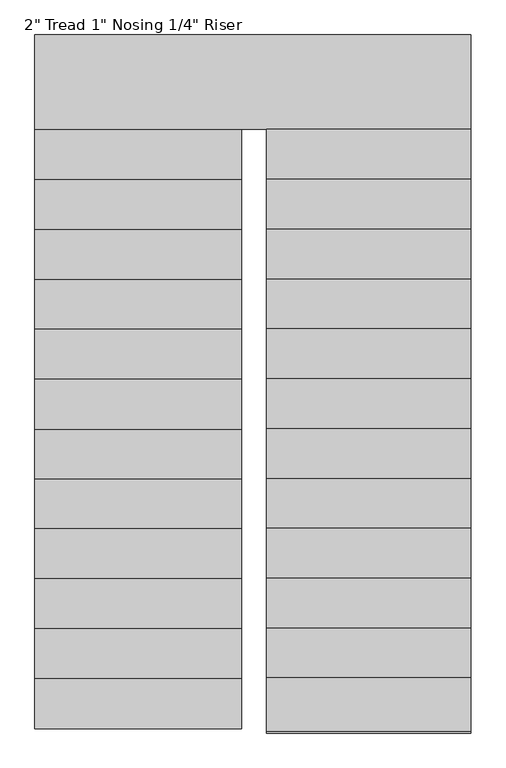
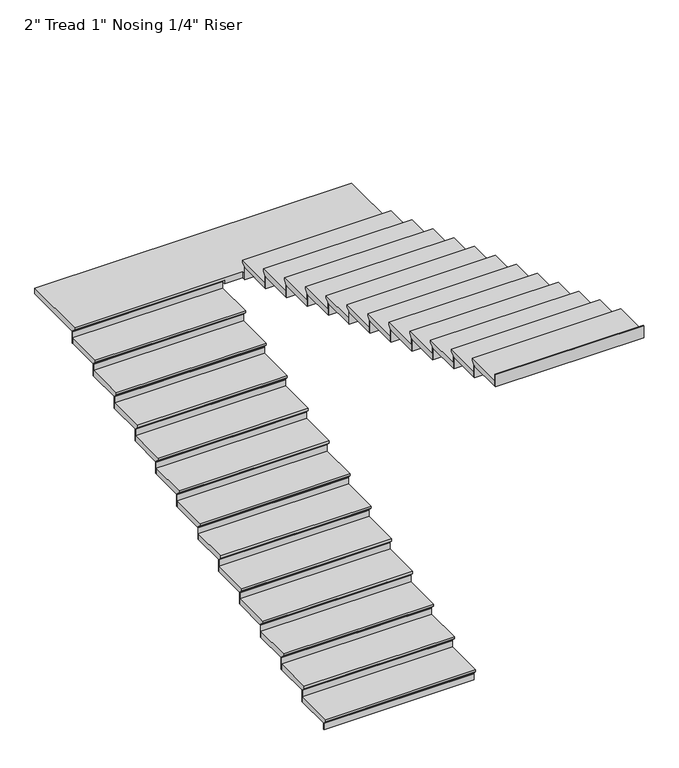
"""IFC4 building model written with IfcOpenShell, lengths in millimetres: stair flight geometry."""

from ifc_helpers import new_model, si_unit, origin, place, context, project, spatial, faceted_brep, source, transform, mapped, element, save


def stair_flight_8b440c70(model_context):
    return source(origin(), model_context, "Body", "Brep", [
        faceted_brep([(-2593.7381751, -9955.5916506, 18374.4576923), (-2593.7381751, -9955.5916506, 18393.5076923), (-3857.687215, -9955.5916506, 18393.5076923), (-3857.687215, -9955.5916506, 18374.4576923), (-2593.7381751, -9930.1916506, 18349.0576923), (-3857.687215, -9930.1916506, 18349.0576923), (-2593.7381751, -9619.0416506, 18393.5076923), (-3857.687215, -9619.0416506, 18393.5076923), (-3857.687215, -9930.1916506, 18342.7076923), (-3857.687215, -9619.0416506, 18342.7076923), (-2593.7381751, -9619.0416506, 18342.7076923), (-2593.7381751, -9930.1916506, 18342.7076923)], [[[0, 1, 2, 3]], [[4, 0, 3, 5]], [[2, 1, 6, 7]], [[8, 9, 10, 11]], [[2, 7, 9, 8, 5, 3]], [[8, 11, 4, 5]], [[6, 1, 0, 4, 11, 10]], [[7, 6, 10, 9]]]),
        faceted_brep([(-2593.7381751, -9930.1916506, 18342.7076923), (-2593.7381751, -9930.1916506, 18288.0), (-2593.7381751, -9923.8416506, 18288.0), (-2593.7381751, -9923.8416506, 18342.7076923), (-3857.687215, -9930.1916506, 18342.7076923), (-3857.687215, -9923.8416506, 18342.7076923), (-3857.687215, -9923.8416506, 18288.0), (-3857.687215, -9930.1916506, 18288.0)], [[[0, 1, 2, 3]], [[4, 5, 6, 7]], [[1, 0, 4, 7]], [[2, 1, 7, 6]], [[3, 2, 6, 5]], [[0, 3, 5, 4]]]),
        faceted_brep([(-2593.7381751, -9619.0416506, 18448.2153846), (-2593.7381751, -9619.0416506, 18342.7076923), (-2593.7381751, -9612.6916506, 18342.7076923), (-2593.7381751, -9612.6916506, 18448.2153846), (-3857.687215, -9619.0416506, 18448.2153846), (-3857.687215, -9612.6916506, 18448.2153846), (-3857.687215, -9612.6916506, 18342.7076923), (-3857.687215, -9619.0416506, 18342.7076923)], [[[0, 1, 2, 3]], [[4, 5, 6, 7]], [[1, 0, 4, 7]], [[2, 1, 7, 6]], [[3, 2, 6, 5]], [[0, 3, 5, 4]]]),
        faceted_brep([(-3857.687215, -9644.4416506, 18499.0153846), (-2593.7381751, -9644.4416506, 18499.0153846), (-2593.7381751, -9314.2416506, 18499.0153846), (-3857.687215, -9314.2416506, 18499.0153846), (-3857.687215, -9619.0416506, 18448.2153846), (-3857.687215, -9314.2416506, 18448.2153846), (-2593.7381751, -9314.2416506, 18448.2153846), (-2593.7381751, -9619.0416506, 18448.2153846), (-3857.687215, -9619.0416506, 18454.5653846), (-3857.687215, -9644.4416506, 18479.9653846), (-2593.7381751, -9619.0416506, 18454.5653846), (-2593.7381751, -9644.4416506, 18479.9653846)], [[[0, 1, 2, 3]], [[4, 5, 6, 7]], [[0, 3, 5, 4, 8, 9]], [[4, 7, 10, 8]], [[2, 1, 11, 10, 7, 6]], [[3, 2, 6, 5]], [[11, 1, 0, 9]], [[10, 11, 9, 8]]]),
        faceted_brep([(-2593.7381751, -9314.2416506, 18553.7230769), (-2593.7381751, -9314.2416506, 18448.2153846), (-2593.7381751, -9307.8916506, 18448.2153846), (-2593.7381751, -9307.8916506, 18553.7230769), (-3857.687215, -9314.2416506, 18553.7230769), (-3857.687215, -9307.8916506, 18553.7230769), (-3857.687215, -9307.8916506, 18448.2153846), (-3857.687215, -9314.2416506, 18448.2153846)], [[[0, 1, 2, 3]], [[4, 5, 6, 7]], [[1, 0, 4, 7]], [[2, 1, 7, 6]], [[3, 2, 6, 5]], [[0, 3, 5, 4]]]),
        faceted_brep([(-3857.687215, -9339.6416506, 18604.5230769), (-2593.7381751, -9339.6416506, 18604.5230769), (-2593.7381751, -9009.4416506, 18604.5230769), (-3857.687215, -9009.4416506, 18604.5230769), (-3857.687215, -9314.2416506, 18553.7230769), (-3857.687215, -9009.4416506, 18553.7230769), (-2593.7381751, -9009.4416506, 18553.7230769), (-2593.7381751, -9314.2416506, 18553.7230769), (-3857.687215, -9314.2416506, 18560.0730769), (-3857.687215, -9339.6416506, 18585.4730769), (-2593.7381751, -9314.2416506, 18560.0730769), (-2593.7381751, -9339.6416506, 18585.4730769)], [[[0, 1, 2, 3]], [[4, 5, 6, 7]], [[0, 3, 5, 4, 8, 9]], [[4, 7, 10, 8]], [[2, 1, 11, 10, 7, 6]], [[3, 2, 6, 5]], [[11, 1, 0, 9]], [[10, 11, 9, 8]]]),
        faceted_brep([(-2593.7381751, -9009.4416506, 18659.2307692), (-2593.7381751, -9009.4416506, 18553.7230769), (-2593.7381751, -9003.0916506, 18553.7230769), (-2593.7381751, -9003.0916506, 18659.2307692), (-3857.687215, -9009.4416506, 18659.2307692), (-3857.687215, -9003.0916506, 18659.2307692), (-3857.687215, -9003.0916506, 18553.7230769), (-3857.687215, -9009.4416506, 18553.7230769)], [[[0, 1, 2, 3]], [[4, 5, 6, 7]], [[1, 0, 4, 7]], [[2, 1, 7, 6]], [[3, 2, 6, 5]], [[0, 3, 5, 4]]]),
        faceted_brep([(-3857.687215, -9034.8416506, 18710.0307692), (-2593.7381751, -9034.8416506, 18710.0307692), (-2593.7381751, -8704.6416506, 18710.0307692), (-3857.687215, -8704.6416506, 18710.0307692), (-3857.687215, -9009.4416506, 18659.2307692), (-3857.687215, -8704.6416506, 18659.2307692), (-2593.7381751, -8704.6416506, 18659.2307692), (-2593.7381751, -9009.4416506, 18659.2307692), (-3857.687215, -9009.4416506, 18665.5807692), (-3857.687215, -9034.8416506, 18690.9807692), (-2593.7381751, -9009.4416506, 18665.5807692), (-2593.7381751, -9034.8416506, 18690.9807692)], [[[0, 1, 2, 3]], [[4, 5, 6, 7]], [[0, 3, 5, 4, 8, 9]], [[4, 7, 10, 8]], [[2, 1, 11, 10, 7, 6]], [[3, 2, 6, 5]], [[11, 1, 0, 9]], [[10, 11, 9, 8]]]),
        faceted_brep([(-2593.7381751, -8704.6416506, 18764.7384615), (-2593.7381751, -8704.6416506, 18659.2307692), (-2593.7381751, -8698.2916506, 18659.2307692), (-2593.7381751, -8698.2916506, 18764.7384615), (-3857.687215, -8704.6416506, 18764.7384615), (-3857.687215, -8698.2916506, 18764.7384615), (-3857.687215, -8698.2916506, 18659.2307692), (-3857.687215, -8704.6416506, 18659.2307692)], [[[0, 1, 2, 3]], [[4, 5, 6, 7]], [[1, 0, 4, 7]], [[2, 1, 7, 6]], [[3, 2, 6, 5]], [[0, 3, 5, 4]]]),
        faceted_brep([(-3857.687215, -8730.0416506, 18815.5384615), (-2593.7381751, -8730.0416506, 18815.5384615), (-2593.7381751, -8399.8416506, 18815.5384615), (-3857.687215, -8399.8416506, 18815.5384615), (-3857.687215, -8704.6416506, 18764.7384615), (-3857.687215, -8399.8416506, 18764.7384615), (-2593.7381751, -8399.8416506, 18764.7384615), (-2593.7381751, -8704.6416506, 18764.7384615), (-3857.687215, -8704.6416506, 18771.0884615), (-3857.687215, -8730.0416506, 18796.4884615), (-2593.7381751, -8704.6416506, 18771.0884615), (-2593.7381751, -8730.0416506, 18796.4884615)], [[[0, 1, 2, 3]], [[4, 5, 6, 7]], [[0, 3, 5, 4, 8, 9]], [[4, 7, 10, 8]], [[2, 1, 11, 10, 7, 6]], [[3, 2, 6, 5]], [[11, 1, 0, 9]], [[10, 11, 9, 8]]]),
        faceted_brep([(-2593.7381751, -8399.8416506, 18870.2461538), (-2593.7381751, -8399.8416506, 18764.7384615), (-2593.7381751, -8393.4916506, 18764.7384615), (-2593.7381751, -8393.4916506, 18870.2461538), (-3857.687215, -8399.8416506, 18870.2461538), (-3857.687215, -8393.4916506, 18870.2461538), (-3857.687215, -8393.4916506, 18764.7384615), (-3857.687215, -8399.8416506, 18764.7384615)], [[[0, 1, 2, 3]], [[4, 5, 6, 7]], [[1, 0, 4, 7]], [[2, 1, 7, 6]], [[3, 2, 6, 5]], [[0, 3, 5, 4]]]),
        faceted_brep([(-3857.687215, -8425.2416506, 18921.0461538), (-2593.7381751, -8425.2416506, 18921.0461538), (-2593.7381751, -8098.2166506, 18921.0461538), (-3857.687215, -8098.2166506, 18921.0461538), (-3857.687215, -8399.8416506, 18870.2461538), (-3857.687215, -8098.2166506, 18870.2461538), (-2593.7381751, -8098.2166506, 18870.2461538), (-2593.7381751, -8399.8416506, 18870.2461538), (-3857.687215, -8399.8416506, 18876.5961538), (-3857.687215, -8425.2416506, 18901.9961538), (-2593.7381751, -8399.8416506, 18876.5961538), (-2593.7381751, -8425.2416506, 18901.9961538)], [[[0, 1, 2, 3]], [[4, 5, 6, 7]], [[0, 3, 5, 4, 8, 9]], [[4, 7, 10, 8]], [[2, 1, 11, 10, 7, 6]], [[3, 2, 6, 5]], [[11, 1, 0, 9]], [[10, 11, 9, 8]]]),
        faceted_brep([(-2593.7381751, -8098.2166506, 18975.7538462), (-2593.7381751, -8098.2166506, 18870.2461538), (-2593.7381751, -8091.8666506, 18870.2461538), (-2593.7381751, -8091.8666506, 18975.7538462), (-3857.687215, -8098.2166506, 18975.7538462), (-3857.687215, -8091.8666506, 18975.7538462), (-3857.687215, -8091.8666506, 18870.2461538), (-3857.687215, -8098.2166506, 18870.2461538)], [[[0, 1, 2, 3]], [[4, 5, 6, 7]], [[1, 0, 4, 7]], [[2, 1, 7, 6]], [[3, 2, 6, 5]], [[0, 3, 5, 4]]]),
        faceted_brep([(-3857.687215, -8123.6166506, 19026.5538462), (-2593.7381751, -8123.6166506, 19026.5538462), (-2593.7381751, -7790.2416506, 19026.5538462), (-3857.687215, -7790.2416506, 19026.5538462), (-3857.687215, -8098.2166506, 18975.7538462), (-3857.687215, -7790.2416506, 18975.7538462), (-2593.7381751, -7790.2416506, 18975.7538462), (-2593.7381751, -8098.2166506, 18975.7538462), (-3857.687215, -8098.2166506, 18982.1038462), (-3857.687215, -8123.6166506, 19007.5038462), (-2593.7381751, -8098.2166506, 18982.1038462), (-2593.7381751, -8123.6166506, 19007.5038462)], [[[0, 1, 2, 3]], [[4, 5, 6, 7]], [[0, 3, 5, 4, 8, 9]], [[4, 7, 10, 8]], [[2, 1, 11, 10, 7, 6]], [[3, 2, 6, 5]], [[11, 1, 0, 9]], [[10, 11, 9, 8]]]),
        faceted_brep([(-2593.7381751, -7790.2416506, 19081.2615385), (-2593.7381751, -7790.2416506, 18975.7538462), (-2593.7381751, -7783.8916506, 18975.7538462), (-2593.7381751, -7783.8916506, 19081.2615385), (-3857.687215, -7790.2416506, 19081.2615385), (-3857.687215, -7783.8916506, 19081.2615385), (-3857.687215, -7783.8916506, 18975.7538462), (-3857.687215, -7790.2416506, 18975.7538462)], [[[0, 1, 2, 3]], [[4, 5, 6, 7]], [[1, 0, 4, 7]], [[2, 1, 7, 6]], [[3, 2, 6, 5]], [[0, 3, 5, 4]]]),
        faceted_brep([(-3857.687215, -7815.6416506, 19132.0615385), (-2593.7381751, -7815.6416506, 19132.0615385), (-2593.7381751, -7485.4416506, 19132.0615385), (-3857.687215, -7485.4416506, 19132.0615385), (-3857.687215, -7790.2416506, 19081.2615385), (-3857.687215, -7485.4416506, 19081.2615385), (-2593.7381751, -7485.4416506, 19081.2615385), (-2593.7381751, -7790.2416506, 19081.2615385), (-3857.687215, -7790.2416506, 19087.6115385), (-3857.687215, -7815.6416506, 19113.0115385), (-2593.7381751, -7790.2416506, 19087.6115385), (-2593.7381751, -7815.6416506, 19113.0115385)], [[[0, 1, 2, 3]], [[4, 5, 6, 7]], [[0, 3, 5, 4, 8, 9]], [[4, 7, 10, 8]], [[2, 1, 11, 10, 7, 6]], [[3, 2, 6, 5]], [[11, 1, 0, 9]], [[10, 11, 9, 8]]]),
        faceted_brep([(-2593.7381751, -7485.4416506, 19186.7692308), (-2593.7381751, -7485.4416506, 19081.2615385), (-2593.7381751, -7479.0916506, 19081.2615385), (-2593.7381751, -7479.0916506, 19186.7692308), (-3857.687215, -7485.4416506, 19186.7692308), (-3857.687215, -7479.0916506, 19186.7692308), (-3857.687215, -7479.0916506, 19081.2615385), (-3857.687215, -7485.4416506, 19081.2615385)], [[[0, 1, 2, 3]], [[4, 5, 6, 7]], [[1, 0, 4, 7]], [[2, 1, 7, 6]], [[3, 2, 6, 5]], [[0, 3, 5, 4]]]),
        faceted_brep([(-3857.687215, -7510.8416506, 19237.5692308), (-2593.7381751, -7510.8416506, 19237.5692308), (-2593.7381751, -7180.6416506, 19237.5692308), (-3857.687215, -7180.6416506, 19237.5692308), (-3857.687215, -7485.4416506, 19186.7692308), (-3857.687215, -7180.6416506, 19186.7692308), (-2593.7381751, -7180.6416506, 19186.7692308), (-2593.7381751, -7485.4416506, 19186.7692308), (-3857.687215, -7485.4416506, 19193.1192308), (-3857.687215, -7510.8416506, 19218.5192308), (-2593.7381751, -7485.4416506, 19193.1192308), (-2593.7381751, -7510.8416506, 19218.5192308)], [[[0, 1, 2, 3]], [[4, 5, 6, 7]], [[0, 3, 5, 4, 8, 9]], [[4, 7, 10, 8]], [[2, 1, 11, 10, 7, 6]], [[3, 2, 6, 5]], [[11, 1, 0, 9]], [[10, 11, 9, 8]]]),
        faceted_brep([(-2593.7381751, -7180.6416506, 19292.2769231), (-2593.7381751, -7180.6416506, 19186.7692308), (-2593.7381751, -7174.2916506, 19186.7692308), (-2593.7381751, -7174.2916506, 19292.2769231), (-3857.687215, -7180.6416506, 19292.2769231), (-3857.687215, -7174.2916506, 19292.2769231), (-3857.687215, -7174.2916506, 19186.7692308), (-3857.687215, -7180.6416506, 19186.7692308)], [[[0, 1, 2, 3]], [[4, 5, 6, 7]], [[1, 0, 4, 7]], [[2, 1, 7, 6]], [[3, 2, 6, 5]], [[0, 3, 5, 4]]]),
        faceted_brep([(-3857.687215, -7206.0416506, 19343.0769231), (-2593.7381751, -7206.0416506, 19343.0769231), (-2593.7381751, -6875.8416506, 19343.0769231), (-3857.687215, -6875.8416506, 19343.0769231), (-3857.687215, -7180.6416506, 19292.2769231), (-3857.687215, -6875.8416506, 19292.2769231), (-2593.7381751, -6875.8416506, 19292.2769231), (-2593.7381751, -7180.6416506, 19292.2769231), (-3857.687215, -7180.6416506, 19298.6269231), (-3857.687215, -7206.0416506, 19324.0269231), (-2593.7381751, -7180.6416506, 19298.6269231), (-2593.7381751, -7206.0416506, 19324.0269231)], [[[0, 1, 2, 3]], [[4, 5, 6, 7]], [[0, 3, 5, 4, 8, 9]], [[4, 7, 10, 8]], [[2, 1, 11, 10, 7, 6]], [[3, 2, 6, 5]], [[11, 1, 0, 9]], [[10, 11, 9, 8]]]),
        faceted_brep([(-2593.7381751, -6875.8416506, 19397.7846154), (-2593.7381751, -6875.8416506, 19292.2769231), (-2593.7381751, -6869.4916506, 19292.2769231), (-2593.7381751, -6869.4916506, 19397.7846154), (-3857.687215, -6875.8416506, 19397.7846154), (-3857.687215, -6869.4916506, 19397.7846154), (-3857.687215, -6869.4916506, 19292.2769231), (-3857.687215, -6875.8416506, 19292.2769231)], [[[0, 1, 2, 3]], [[4, 5, 6, 7]], [[1, 0, 4, 7]], [[2, 1, 7, 6]], [[3, 2, 6, 5]], [[0, 3, 5, 4]]]),
        faceted_brep([(-3857.687215, -6901.2416506, 19448.5846154), (-2593.7381751, -6901.2416506, 19448.5846154), (-2593.7381751, -6571.0416506, 19448.5846154), (-3857.687215, -6571.0416506, 19448.5846154), (-3857.687215, -6875.8416506, 19397.7846154), (-3857.687215, -6571.0416506, 19397.7846154), (-2593.7381751, -6571.0416506, 19397.7846154), (-2593.7381751, -6875.8416506, 19397.7846154), (-3857.687215, -6875.8416506, 19404.1346154), (-3857.687215, -6901.2416506, 19429.5346154), (-2593.7381751, -6875.8416506, 19404.1346154), (-2593.7381751, -6901.2416506, 19429.5346154)], [[[0, 1, 2, 3]], [[4, 5, 6, 7]], [[0, 3, 5, 4, 8, 9]], [[4, 7, 10, 8]], [[2, 1, 11, 10, 7, 6]], [[3, 2, 6, 5]], [[11, 1, 0, 9]], [[10, 11, 9, 8]]]),
        faceted_brep([(-2593.7381751, -6571.0416506, 19503.2923077), (-2593.7381751, -6571.0416506, 19397.7846154), (-2593.7381751, -6564.6916506, 19397.7846154), (-2593.7381751, -6564.6916506, 19503.2923077), (-3857.687215, -6571.0416506, 19503.2923077), (-3857.687215, -6564.6916506, 19503.2923077), (-3857.687215, -6564.6916506, 19397.7846154), (-3857.687215, -6571.0416506, 19397.7846154)], [[[0, 1, 2, 3]], [[4, 5, 6, 7]], [[1, 0, 4, 7]], [[2, 1, 7, 6]], [[3, 2, 6, 5]], [[0, 3, 5, 4]]]),
        faceted_brep([(-3857.687215, -6596.4416506, 19554.0923077), (-2593.7381751, -6596.4416506, 19554.0923077), (-2593.7381751, -6266.2416506, 19554.0923077), (-3857.687215, -6266.2416506, 19554.0923077), (-3857.687215, -6571.0416506, 19503.2923077), (-3857.687215, -6266.2416506, 19503.2923077), (-2593.7381751, -6266.2416506, 19503.2923077), (-2593.7381751, -6571.0416506, 19503.2923077), (-3857.687215, -6571.0416506, 19509.6423077), (-3857.687215, -6596.4416506, 19535.0423077), (-2593.7381751, -6571.0416506, 19509.6423077), (-2593.7381751, -6596.4416506, 19535.0423077)], [[[0, 1, 2, 3]], [[4, 5, 6, 7]], [[0, 3, 5, 4, 8, 9]], [[4, 7, 10, 8]], [[2, 1, 11, 10, 7, 6]], [[3, 2, 6, 5]], [[11, 1, 0, 9]], [[10, 11, 9, 8]]]),
        faceted_brep([(-2593.7381751, -6266.2416506, 19608.8), (-2593.7381751, -6266.2416506, 19503.2923077), (-2593.7381751, -6259.8916506, 19503.2923077), (-2593.7381751, -6259.8916506, 19608.8), (-3857.687215, -6266.2416506, 19608.8), (-3857.687215, -6259.8916506, 19608.8), (-3857.687215, -6259.8916506, 19503.2923077), (-3857.687215, -6266.2416506, 19503.2923077)], [[[0, 1, 2, 3]], [[4, 5, 6, 7]], [[1, 0, 4, 7]], [[2, 1, 7, 6]], [[3, 2, 6, 5]], [[0, 3, 5, 4]]]),
        faceted_brep([(-1190.687215, -6317.0416506, 19659.6), (-1190.687215, -5713.7916506, 19659.6), (-3857.687215, -5713.7916506, 19659.6), (-3857.687215, -6291.6416506, 19659.6), (-2441.3381751, -6291.6416506, 19659.6), (-2441.3381751, -6317.0416506, 19659.6), (-1190.687215, -5713.7916506, 19608.8), (-1190.687215, -6317.0416506, 19608.8), (-2441.3381751, -6317.0416506, 19608.8), (-2441.3381751, -6291.6416506, 19608.8), (-2593.7381751, -6291.6416506, 19608.8), (-2593.7381751, -6266.2416506, 19608.8), (-3857.687215, -6266.2416506, 19608.8), (-3857.687215, -5713.7916506, 19608.8), (-3857.687215, -6266.2416506, 19615.15), (-3857.687215, -6291.6416506, 19640.55), (-2593.7381751, -6266.2416506, 19615.15), (-2593.7381751, -6291.6416506, 19640.55)], [[[0, 1, 2, 3, 4, 5]], [[6, 7, 8, 9, 10, 11, 12, 13]], [[1, 0, 7, 6]], [[2, 1, 6, 13]], [[3, 2, 13, 12, 14, 15]], [[12, 11, 16, 14]], [[11, 10, 17, 16]], [[4, 3, 15, 17, 10, 9]], [[5, 4, 9, 8]], [[0, 5, 8, 7]], [[15, 14, 16, 17]]]),
        faceted_brep([(-2441.3381751, -6317.0416506, 19714.3076923), (-2441.3381751, -6317.0416506, 19608.8), (-2441.3381751, -6323.3916506, 19608.8), (-2441.3381751, -6323.3916506, 19714.3076923), (-1190.687215, -6317.0416506, 19714.3076923), (-1190.687215, -6323.3916506, 19714.3076923), (-1190.687215, -6323.3916506, 19608.8), (-1190.687215, -6317.0416506, 19608.8)], [[[0, 1, 2, 3]], [[4, 5, 6, 7]], [[1, 0, 4, 7]], [[2, 1, 7, 6]], [[3, 2, 6, 5]], [[0, 3, 5, 4]]]),
        faceted_brep([(-1190.687215, -6291.6416506, 19765.1076923), (-2441.3381751, -6291.6416506, 19765.1076923), (-2441.3381751, -6621.8416506, 19765.1076923), (-1190.687215, -6621.8416506, 19765.1076923), (-1190.687215, -6317.0416506, 19714.3076923), (-1190.687215, -6621.8416506, 19714.3076923), (-2441.3381751, -6621.8416506, 19714.3076923), (-2441.3381751, -6317.0416506, 19714.3076923), (-1190.687215, -6317.0416506, 19720.6576923), (-1190.687215, -6291.6416506, 19746.0576923), (-2441.3381751, -6317.0416506, 19720.6576923), (-2441.3381751, -6291.6416506, 19746.0576923)], [[[0, 1, 2, 3]], [[4, 5, 6, 7]], [[0, 3, 5, 4, 8, 9]], [[4, 7, 10, 8]], [[2, 1, 11, 10, 7, 6]], [[3, 2, 6, 5]], [[11, 1, 0, 9]], [[10, 11, 9, 8]]]),
        faceted_brep([(-2441.3381751, -6621.8416506, 19819.8153846), (-2441.3381751, -6621.8416506, 19714.3076923), (-2441.3381751, -6628.1916506, 19714.3076923), (-2441.3381751, -6628.1916506, 19819.8153846), (-1190.687215, -6621.8416506, 19819.8153846), (-1190.687215, -6628.1916506, 19819.8153846), (-1190.687215, -6628.1916506, 19714.3076923), (-1190.687215, -6621.8416506, 19714.3076923)], [[[0, 1, 2, 3]], [[4, 5, 6, 7]], [[1, 0, 4, 7]], [[2, 1, 7, 6]], [[3, 2, 6, 5]], [[0, 3, 5, 4]]]),
        faceted_brep([(-1190.687215, -6596.4416506, 19870.6153846), (-2441.3381751, -6596.4416506, 19870.6153846), (-2441.3381751, -6926.6416506, 19870.6153846), (-1190.687215, -6926.6416506, 19870.6153846), (-1190.687215, -6621.8416506, 19819.8153846), (-1190.687215, -6926.6416506, 19819.8153846), (-2441.3381751, -6926.6416506, 19819.8153846), (-2441.3381751, -6621.8416506, 19819.8153846), (-1190.687215, -6621.8416506, 19826.1653846), (-1190.687215, -6596.4416506, 19851.5653846), (-2441.3381751, -6621.8416506, 19826.1653846), (-2441.3381751, -6596.4416506, 19851.5653846)], [[[0, 1, 2, 3]], [[4, 5, 6, 7]], [[0, 3, 5, 4, 8, 9]], [[4, 7, 10, 8]], [[2, 1, 11, 10, 7, 6]], [[3, 2, 6, 5]], [[11, 1, 0, 9]], [[10, 11, 9, 8]]]),
        faceted_brep([(-2441.3381751, -6926.6416506, 19925.3230769), (-2441.3381751, -6926.6416506, 19819.8153846), (-2441.3381751, -6932.9916506, 19819.8153846), (-2441.3381751, -6932.9916506, 19925.3230769), (-1190.687215, -6926.6416506, 19925.3230769), (-1190.687215, -6932.9916506, 19925.3230769), (-1190.687215, -6932.9916506, 19819.8153846), (-1190.687215, -6926.6416506, 19819.8153846)], [[[0, 1, 2, 3]], [[4, 5, 6, 7]], [[1, 0, 4, 7]], [[2, 1, 7, 6]], [[3, 2, 6, 5]], [[0, 3, 5, 4]]]),
        faceted_brep([(-1190.687215, -6901.2416506, 19976.1230769), (-2441.3381751, -6901.2416506, 19976.1230769), (-2441.3381751, -7231.4416506, 19976.1230769), (-1190.687215, -7231.4416506, 19976.1230769), (-1190.687215, -6926.6416506, 19925.3230769), (-1190.687215, -7231.4416506, 19925.3230769), (-2441.3381751, -7231.4416506, 19925.3230769), (-2441.3381751, -6926.6416506, 19925.3230769), (-1190.687215, -6926.6416506, 19931.6730769), (-1190.687215, -6901.2416506, 19957.0730769), (-2441.3381751, -6926.6416506, 19931.6730769), (-2441.3381751, -6901.2416506, 19957.0730769)], [[[0, 1, 2, 3]], [[4, 5, 6, 7]], [[0, 3, 5, 4, 8, 9]], [[4, 7, 10, 8]], [[2, 1, 11, 10, 7, 6]], [[3, 2, 6, 5]], [[11, 1, 0, 9]], [[10, 11, 9, 8]]]),
        faceted_brep([(-2441.3381751, -7231.4416506, 20030.8307692), (-2441.3381751, -7231.4416506, 19925.3230769), (-2441.3381751, -7237.7916506, 19925.3230769), (-2441.3381751, -7237.7916506, 20030.8307692), (-1190.687215, -7231.4416506, 20030.8307692), (-1190.687215, -7237.7916506, 20030.8307692), (-1190.687215, -7237.7916506, 19925.3230769), (-1190.687215, -7231.4416506, 19925.3230769)], [[[0, 1, 2, 3]], [[4, 5, 6, 7]], [[1, 0, 4, 7]], [[2, 1, 7, 6]], [[3, 2, 6, 5]], [[0, 3, 5, 4]]]),
        faceted_brep([(-1190.687215, -7206.0416506, 20081.6307692), (-2441.3381751, -7206.0416506, 20081.6307692), (-2441.3381751, -7536.2416506, 20081.6307692), (-1190.687215, -7536.2416506, 20081.6307692), (-1190.687215, -7231.4416506, 20030.8307692), (-1190.687215, -7536.2416506, 20030.8307692), (-2441.3381751, -7536.2416506, 20030.8307692), (-2441.3381751, -7231.4416506, 20030.8307692), (-1190.687215, -7231.4416506, 20037.1807692), (-1190.687215, -7206.0416506, 20062.5807692), (-2441.3381751, -7231.4416506, 20037.1807692), (-2441.3381751, -7206.0416506, 20062.5807692)], [[[0, 1, 2, 3]], [[4, 5, 6, 7]], [[0, 3, 5, 4, 8, 9]], [[4, 7, 10, 8]], [[2, 1, 11, 10, 7, 6]], [[3, 2, 6, 5]], [[11, 1, 0, 9]], [[10, 11, 9, 8]]]),
        faceted_brep([(-2441.3381751, -7536.2416506, 20136.3384615), (-2441.3381751, -7536.2416506, 20030.8307692), (-2441.3381751, -7542.5916506, 20030.8307692), (-2441.3381751, -7542.5916506, 20136.3384615), (-1190.687215, -7536.2416506, 20136.3384615), (-1190.687215, -7542.5916506, 20136.3384615), (-1190.687215, -7542.5916506, 20030.8307692), (-1190.687215, -7536.2416506, 20030.8307692)], [[[0, 1, 2, 3]], [[4, 5, 6, 7]], [[1, 0, 4, 7]], [[2, 1, 7, 6]], [[3, 2, 6, 5]], [[0, 3, 5, 4]]]),
        faceted_brep([(-1190.687215, -7510.8416506, 20187.1384615), (-2441.3381751, -7510.8416506, 20187.1384615), (-2441.3381751, -7841.0416506, 20187.1384615), (-1190.687215, -7841.0416506, 20187.1384615), (-1190.687215, -7536.2416506, 20136.3384615), (-1190.687215, -7841.0416506, 20136.3384615), (-2441.3381751, -7841.0416506, 20136.3384615), (-2441.3381751, -7536.2416506, 20136.3384615), (-1190.687215, -7536.2416506, 20142.6884615), (-1190.687215, -7510.8416506, 20168.0884615), (-2441.3381751, -7536.2416506, 20142.6884615), (-2441.3381751, -7510.8416506, 20168.0884615)], [[[0, 1, 2, 3]], [[4, 5, 6, 7]], [[0, 3, 5, 4, 8, 9]], [[4, 7, 10, 8]], [[2, 1, 11, 10, 7, 6]], [[3, 2, 6, 5]], [[11, 1, 0, 9]], [[10, 11, 9, 8]]]),
        faceted_brep([(-2441.3381751, -7841.0416506, 20241.8461538), (-2441.3381751, -7841.0416506, 20136.3384615), (-2441.3381751, -7847.3916506, 20136.3384615), (-2441.3381751, -7847.3916506, 20241.8461538), (-1190.687215, -7841.0416506, 20241.8461538), (-1190.687215, -7847.3916506, 20241.8461538), (-1190.687215, -7847.3916506, 20136.3384615), (-1190.687215, -7841.0416506, 20136.3384615)], [[[0, 1, 2, 3]], [[4, 5, 6, 7]], [[1, 0, 4, 7]], [[2, 1, 7, 6]], [[3, 2, 6, 5]], [[0, 3, 5, 4]]]),
        faceted_brep([(-1190.687215, -7815.6416506, 20292.6461538), (-2441.3381751, -7815.6416506, 20292.6461538), (-2441.3381751, -8145.8416506, 20292.6461538), (-1190.687215, -8145.8416506, 20292.6461538), (-1190.687215, -7841.0416506, 20241.8461538), (-1190.687215, -8145.8416506, 20241.8461538), (-2441.3381751, -8145.8416506, 20241.8461538), (-2441.3381751, -7841.0416506, 20241.8461538), (-1190.687215, -7841.0416506, 20248.1961538), (-1190.687215, -7815.6416506, 20273.5961538), (-2441.3381751, -7841.0416506, 20248.1961538), (-2441.3381751, -7815.6416506, 20273.5961538)], [[[0, 1, 2, 3]], [[4, 5, 6, 7]], [[0, 3, 5, 4, 8, 9]], [[4, 7, 10, 8]], [[2, 1, 11, 10, 7, 6]], [[3, 2, 6, 5]], [[11, 1, 0, 9]], [[10, 11, 9, 8]]]),
        faceted_brep([(-2441.3381751, -8145.8416506, 20347.3538462), (-2441.3381751, -8145.8416506, 20241.8461538), (-2441.3381751, -8152.1916506, 20241.8461538), (-2441.3381751, -8152.1916506, 20347.3538462), (-1190.687215, -8145.8416506, 20347.3538462), (-1190.687215, -8152.1916506, 20347.3538462), (-1190.687215, -8152.1916506, 20241.8461538), (-1190.687215, -8145.8416506, 20241.8461538)], [[[0, 1, 2, 3]], [[4, 5, 6, 7]], [[1, 0, 4, 7]], [[2, 1, 7, 6]], [[3, 2, 6, 5]], [[0, 3, 5, 4]]]),
        faceted_brep([(-1190.687215, -8120.4416506, 20398.1538462), (-2441.3381751, -8120.4416506, 20398.1538462), (-2441.3381751, -8450.6416506, 20398.1538462), (-1190.687215, -8450.6416506, 20398.1538462), (-1190.687215, -8145.8416506, 20347.3538462), (-1190.687215, -8450.6416506, 20347.3538462), (-2441.3381751, -8450.6416506, 20347.3538462), (-2441.3381751, -8145.8416506, 20347.3538462), (-1190.687215, -8145.8416506, 20353.7038462), (-1190.687215, -8120.4416506, 20379.1038462), (-2441.3381751, -8145.8416506, 20353.7038462), (-2441.3381751, -8120.4416506, 20379.1038462)], [[[0, 1, 2, 3]], [[4, 5, 6, 7]], [[0, 3, 5, 4, 8, 9]], [[4, 7, 10, 8]], [[2, 1, 11, 10, 7, 6]], [[3, 2, 6, 5]], [[11, 1, 0, 9]], [[10, 11, 9, 8]]]),
        faceted_brep([(-2441.3381751, -8450.6416506, 20452.8615385), (-2441.3381751, -8450.6416506, 20347.3538462), (-2441.3381751, -8456.9916506, 20347.3538462), (-2441.3381751, -8456.9916506, 20452.8615385), (-1190.687215, -8450.6416506, 20452.8615385), (-1190.687215, -8456.9916506, 20452.8615385), (-1190.687215, -8456.9916506, 20347.3538462), (-1190.687215, -8450.6416506, 20347.3538462)], [[[0, 1, 2, 3]], [[4, 5, 6, 7]], [[1, 0, 4, 7]], [[2, 1, 7, 6]], [[3, 2, 6, 5]], [[0, 3, 5, 4]]]),
        faceted_brep([(-1190.687215, -8425.2416506, 20503.6615385), (-2441.3381751, -8425.2416506, 20503.6615385), (-2441.3381751, -8755.4416506, 20503.6615385), (-1190.687215, -8755.4416506, 20503.6615385), (-1190.687215, -8450.6416506, 20452.8615385), (-1190.687215, -8755.4416506, 20452.8615385), (-2441.3381751, -8755.4416506, 20452.8615385), (-2441.3381751, -8450.6416506, 20452.8615385), (-1190.687215, -8450.6416506, 20459.2115385), (-1190.687215, -8425.2416506, 20484.6115385), (-2441.3381751, -8450.6416506, 20459.2115385), (-2441.3381751, -8425.2416506, 20484.6115385)], [[[0, 1, 2, 3]], [[4, 5, 6, 7]], [[0, 3, 5, 4, 8, 9]], [[4, 7, 10, 8]], [[2, 1, 11, 10, 7, 6]], [[3, 2, 6, 5]], [[11, 1, 0, 9]], [[10, 11, 9, 8]]]),
        faceted_brep([(-2441.3381751, -8755.4416506, 20558.3692308), (-2441.3381751, -8755.4416506, 20452.8615385), (-2441.3381751, -8761.7916506, 20452.8615385), (-2441.3381751, -8761.7916506, 20558.3692308), (-1190.687215, -8755.4416506, 20558.3692308), (-1190.687215, -8761.7916506, 20558.3692308), (-1190.687215, -8761.7916506, 20452.8615385), (-1190.687215, -8755.4416506, 20452.8615385)], [[[0, 1, 2, 3]], [[4, 5, 6, 7]], [[1, 0, 4, 7]], [[2, 1, 7, 6]], [[3, 2, 6, 5]], [[0, 3, 5, 4]]]),
        faceted_brep([(-1190.687215, -8730.0416506, 20609.1692308), (-2441.3381751, -8730.0416506, 20609.1692308), (-2441.3381751, -9060.2416506, 20609.1692308), (-1190.687215, -9060.2416506, 20609.1692308), (-1190.687215, -8755.4416506, 20558.3692308), (-1190.687215, -9060.2416506, 20558.3692308), (-2441.3381751, -9060.2416506, 20558.3692308), (-2441.3381751, -8755.4416506, 20558.3692308), (-1190.687215, -8755.4416506, 20564.7192308), (-1190.687215, -8730.0416506, 20590.1192308), (-2441.3381751, -8755.4416506, 20564.7192308), (-2441.3381751, -8730.0416506, 20590.1192308)], [[[0, 1, 2, 3]], [[4, 5, 6, 7]], [[0, 3, 5, 4, 8, 9]], [[4, 7, 10, 8]], [[2, 1, 11, 10, 7, 6]], [[3, 2, 6, 5]], [[11, 1, 0, 9]], [[10, 11, 9, 8]]]),
        faceted_brep([(-2441.3381751, -9060.2416506, 20663.8769231), (-2441.3381751, -9060.2416506, 20558.3692308), (-2441.3381751, -9066.5916506, 20558.3692308), (-2441.3381751, -9066.5916506, 20663.8769231), (-1190.687215, -9060.2416506, 20663.8769231), (-1190.687215, -9066.5916506, 20663.8769231), (-1190.687215, -9066.5916506, 20558.3692308), (-1190.687215, -9060.2416506, 20558.3692308)], [[[0, 1, 2, 3]], [[4, 5, 6, 7]], [[1, 0, 4, 7]], [[2, 1, 7, 6]], [[3, 2, 6, 5]], [[0, 3, 5, 4]]]),
        faceted_brep([(-1190.687215, -9034.8416506, 20714.6769231), (-2441.3381751, -9034.8416506, 20714.6769231), (-2441.3381751, -9365.0416506, 20714.6769231), (-1190.687215, -9365.0416506, 20714.6769231), (-1190.687215, -9060.2416506, 20663.8769231), (-1190.687215, -9365.0416506, 20663.8769231), (-2441.3381751, -9365.0416506, 20663.8769231), (-2441.3381751, -9060.2416506, 20663.8769231), (-1190.687215, -9060.2416506, 20670.2269231), (-1190.687215, -9034.8416506, 20695.6269231), (-2441.3381751, -9060.2416506, 20670.2269231), (-2441.3381751, -9034.8416506, 20695.6269231)], [[[0, 1, 2, 3]], [[4, 5, 6, 7]], [[0, 3, 5, 4, 8, 9]], [[4, 7, 10, 8]], [[2, 1, 11, 10, 7, 6]], [[3, 2, 6, 5]], [[11, 1, 0, 9]], [[10, 11, 9, 8]]]),
        faceted_brep([(-2441.3381751, -9365.0416506, 20769.3846154), (-2441.3381751, -9365.0416506, 20663.8769231), (-2441.3381751, -9371.3916506, 20663.8769231), (-2441.3381751, -9371.3916506, 20769.3846154), (-1190.687215, -9365.0416506, 20769.3846154), (-1190.687215, -9371.3916506, 20769.3846154), (-1190.687215, -9371.3916506, 20663.8769231), (-1190.687215, -9365.0416506, 20663.8769231)], [[[0, 1, 2, 3]], [[4, 5, 6, 7]], [[1, 0, 4, 7]], [[2, 1, 7, 6]], [[3, 2, 6, 5]], [[0, 3, 5, 4]]]),
        faceted_brep([(-1190.687215, -9339.6416506, 20820.1846154), (-2441.3381751, -9339.6416506, 20820.1846154), (-2441.3381751, -9669.8416506, 20820.1846154), (-1190.687215, -9669.8416506, 20820.1846154), (-1190.687215, -9365.0416506, 20769.3846154), (-1190.687215, -9669.8416506, 20769.3846154), (-2441.3381751, -9669.8416506, 20769.3846154), (-2441.3381751, -9365.0416506, 20769.3846154), (-1190.687215, -9365.0416506, 20775.7346154), (-1190.687215, -9339.6416506, 20801.1346154), (-2441.3381751, -9365.0416506, 20775.7346154), (-2441.3381751, -9339.6416506, 20801.1346154)], [[[0, 1, 2, 3]], [[4, 5, 6, 7]], [[0, 3, 5, 4, 8, 9]], [[4, 7, 10, 8]], [[2, 1, 11, 10, 7, 6]], [[3, 2, 6, 5]], [[11, 1, 0, 9]], [[10, 11, 9, 8]]]),
        faceted_brep([(-2441.3381751, -9669.8416506, 20874.8923077), (-2441.3381751, -9669.8416506, 20769.3846154), (-2441.3381751, -9676.1916506, 20769.3846154), (-2441.3381751, -9676.1916506, 20874.8923077), (-1190.687215, -9669.8416506, 20874.8923077), (-1190.687215, -9676.1916506, 20874.8923077), (-1190.687215, -9676.1916506, 20769.3846154), (-1190.687215, -9669.8416506, 20769.3846154)], [[[0, 1, 2, 3]], [[4, 5, 6, 7]], [[1, 0, 4, 7]], [[2, 1, 7, 6]], [[3, 2, 6, 5]], [[0, 3, 5, 4]]]),
        faceted_brep([(-2441.3381751, -9974.6416506, 20980.4), (-2441.3381751, -9974.6416506, 20874.8923077), (-2441.3381751, -9980.9916506, 20874.8923077), (-2441.3381751, -9980.9916506, 20980.4), (-1190.687215, -9974.6416506, 20980.4), (-1190.687215, -9980.9916506, 20980.4), (-1190.687215, -9980.9916506, 20874.8923077), (-1190.687215, -9974.6416506, 20874.8923077)], [[[0, 1, 2, 3]], [[4, 5, 6, 7]], [[1, 0, 4, 7]], [[2, 1, 7, 6]], [[3, 2, 6, 5]], [[0, 3, 5, 4]]]),
        faceted_brep([(-1190.687215, -9644.4416506, 20925.6923077), (-2441.3381751, -9644.4416506, 20925.6923077), (-2441.3381751, -9974.6416506, 20925.6923077), (-1190.687215, -9974.6416506, 20925.6923077), (-1190.687215, -9669.8416506, 20874.8923077), (-1190.687215, -9974.6416506, 20874.8923077), (-2441.3381751, -9974.6416506, 20874.8923077), (-2441.3381751, -9669.8416506, 20874.8923077), (-1190.687215, -9669.8416506, 20881.2423077), (-1190.687215, -9644.4416506, 20906.6423077), (-2441.3381751, -9669.8416506, 20881.2423077), (-2441.3381751, -9644.4416506, 20906.6423077)], [[[0, 1, 2, 3]], [[4, 5, 6, 7]], [[0, 3, 5, 4, 8, 9]], [[4, 7, 10, 8]], [[2, 1, 11, 10, 7, 6]], [[3, 2, 6, 5]], [[11, 1, 0, 9]], [[10, 11, 9, 8]]]),
    ])


if __name__ == "__main__":
    model = new_model("IFC4")
    model_context = context("Model", 3, world=origin())
    ifc_project = project(units=[si_unit("LENGTHUNIT", "METRE", prefix="MILLI")], contexts=[model_context])
    site = spatial("IfcSite", under=ifc_project)
    building = spatial("IfcBuilding", under=site)
    placement = place(None, origin())
    stair_flight_shape = stair_flight_8b440c70(model_context)
    element("IfcStairFlight", 1, ObjectType="2\" Tread 1\" Nosing 1/4\" Riser", at=placement, inside=building, context=model_context, shape_type="MappedRepresentation", body=[
        mapped(stair_flight_shape, transform((0.0, 0.0, 0.0), x_axis=(1.0, 0.0, 0.0), y_axis=(0.0, 1.0, 0.0), z_axis=(0.0, 0.0, 1.0))),
    ])
    save(model, "model.ifc")
